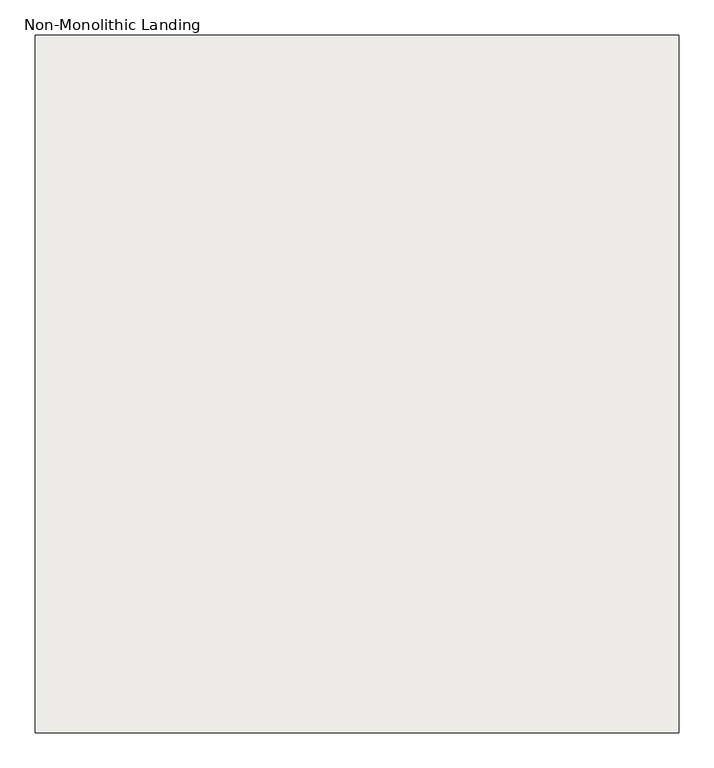
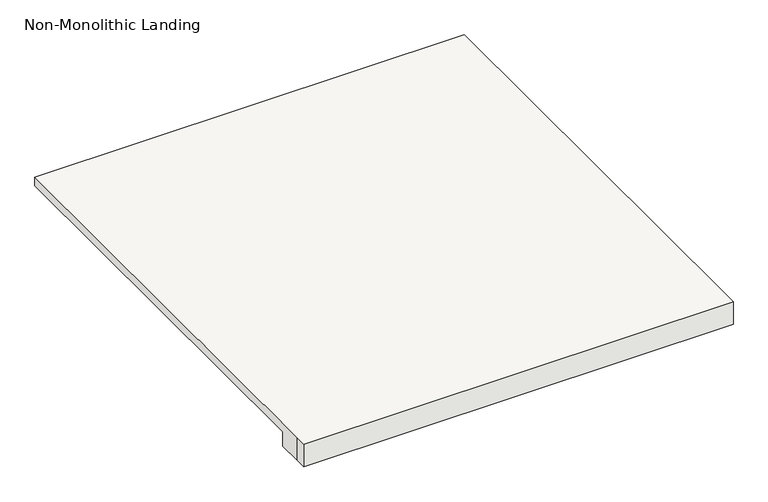
"""IFC4 building model written with IfcOpenShell, lengths in millimetres: slab geometry, Non-Monolithic Landing."""

from ifc_helpers import new_model, si_unit, origin, place, context, project, spatial, faceted_brep, source, transform, mapped, element, save


def non_monolithic_landing_245f9fea(model_context):
    return source(origin(), model_context, "Body", "Brep", [
        faceted_brep([(-803.1608498, 4479.7115866, 1166.2833333), (-777.7608498, 4479.7115866, 1140.8833333), (-777.7608498, 3565.3115866, 1140.8833333), (-803.1608498, 3565.3115866, 1166.2833333), (-803.1608498, 3514.5115866, 1185.3333333), (-803.1608498, 3489.1115866, 1185.3333333), (111.2391502, 3489.1115866, 1185.3333333), (111.2391502, 3514.5115866, 1185.3333333), (111.2391502, 4479.7115866, 1185.3333333), (-803.1608498, 4479.7115866, 1185.3333333), (-777.7608498, 3565.3115866, 1134.5333333), (-777.7608498, 4479.7115866, 1134.5333333), (111.2391502, 4479.7115866, 1134.5333333), (111.2391502, 3514.5115866, 1134.5333333), (111.2391502, 3489.1115866, 1134.5333333), (-803.1608498, 3489.1115866, 1134.5333333), (-803.1608498, 3514.5115866, 1134.5333333), (-803.1608498, 3565.3115866, 1134.5333333)], [[[0, 1, 2, 3]], [[4, 5, 6, 7, 8, 9]], [[10, 11, 12, 13, 14, 15, 16, 17]], [[11, 10, 2, 1]], [[10, 17, 3, 2]], [[4, 9, 0, 3, 17, 16]], [[5, 4, 16, 15]], [[6, 5, 15, 14]], [[7, 6, 14, 13]], [[8, 7, 13, 12]], [[9, 8, 12, 11, 1, 0]]]),
    ])


if __name__ == "__main__":
    model = new_model("IFC4")
    model_context = context("Model", 3, world=origin())
    ifc_project = project(units=[si_unit("LENGTHUNIT", "METRE", prefix="MILLI")], contexts=[model_context])
    site = spatial("IfcSite", under=ifc_project)
    building = spatial("IfcBuilding", under=site)
    placement = place(None, origin())
    non_monolithic_landing_shape = non_monolithic_landing_245f9fea(model_context)
    element("IfcSlab", 1, ObjectType="Non-Monolithic Landing", at=placement, inside=building, context=model_context, shape_type="MappedRepresentation", body=[
        mapped(non_monolithic_landing_shape, transform((0.0, 0.0, 0.0), x_axis=(1.0, 0.0, 0.0), y_axis=(0.0, 1.0, 0.0), z_axis=(0.0, 0.0, 1.0))),
    ])
    save(model, "model.ifc")
